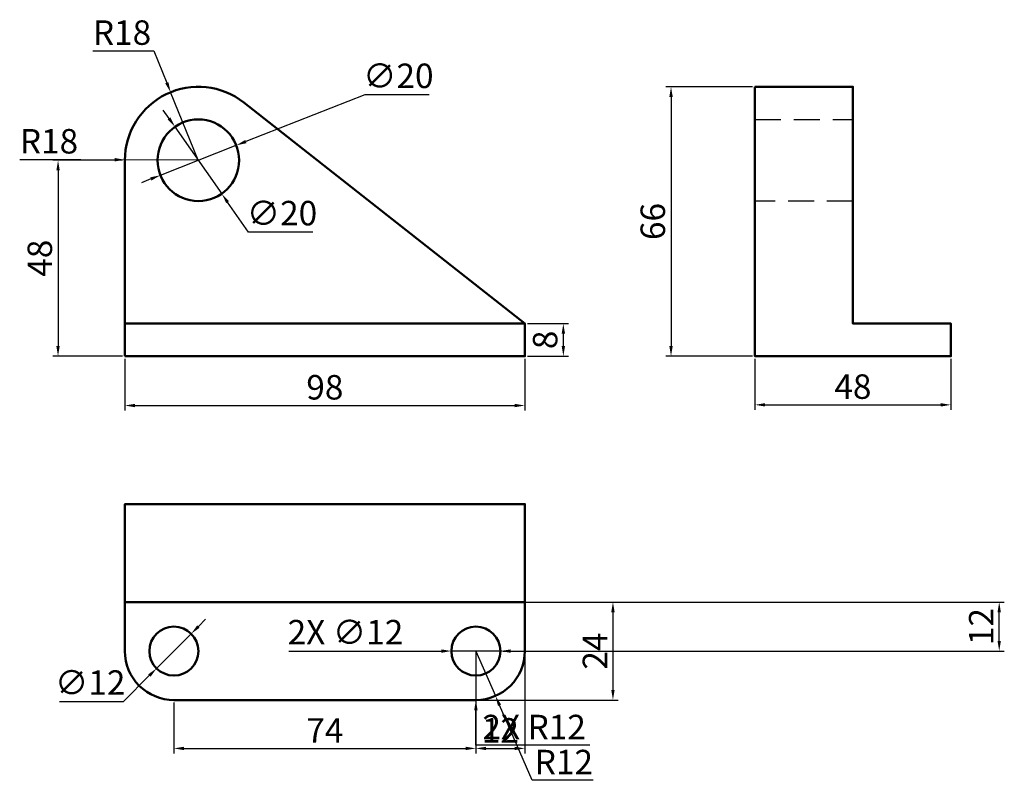
# Model space of a CAD drawing. Units: millimetres. Extents: x 6 to 247, y 96 to 282.
import ezdxf

# ---------------------------------------------------------------- set-up
doc = ezdxf.new("R2010")
doc.units = ezdxf.units.MM
doc.linetypes.add('HIDDEN', pattern=[9.525, 6.35, -3.175])
for name, color, linetype, lineweight in [('M-DIMS', 2, 'Continuous', 25), ('M-HIDN', 3, 'HIDDEN', 25), ('M-OUTL', 7, 'Continuous', 50)]:
    doc.layers.add(name, color=color, linetype=linetype, lineweight=lineweight)
doc.styles.get("Standard").update_dxf_attribs({"font": 'arial.ttf'})
doc.dimstyles.new('ISO-25', dxfattribs={"dimtxt": 6, "dimasz": 2.5, "dimexe": 1.25, "dimexo": 0.625, "dimtad": 1, "dimtoh": 1, "dimdec": 0, "dimtxsty": 'Standard', "dimcen": 2.5, "dimadec": 0, "dimazin": 0, "dimtfac": 1, "dimtdec": 0, "dimtmove": 0, "dimatfit": 3, "dimfxl": 1, "dimarcsym": 0})

# ---------------------------------------------------------------- blocks, each defined once
blk = doc.blocks.new('*D1')
at = {"layer": 'Defpoints', "color": 0, "transparency": 16777216}
for p in [(31.61, 247.68), (15.24, 199.68), (31.61, 199.68)]:
    blk.add_point(p, dxfattribs=at)
at = {"layer": 'M-DIMS', "color": 0, "lineweight": -2, "transparency": 16777216}
for p, q in [((30.99, 247.68), (13.99, 247.68)), ((15.24, 245.18), (15.24, 202.18)), ((30.99, 199.68), (13.99, 199.68))]:
    blk.add_line(p, q, dxfattribs=at)
at = {"layer": 'M-DIMS', "color": 0, "transparency": 16777216}
for points in [[(14.82, 245.18), (15.65, 245.18), (15.24, 247.68)], [(14.82, 202.18), (15.65, 202.18), (15.24, 199.68)]]:
    blk.add_solid(points, dxfattribs=at)
at = {"layer": 'M-DIMS', "color": 0, "transparency": 16777216, "insert": (11.55, 223.68), "char_height": 6, "attachment_point": 5, "rotation": 90}
blk.add_mtext('48', dxfattribs=at)
blk = doc.blocks.new('*D2')
at = {"layer": 'Defpoints', "color": 0, "transparency": 16777216}
for p in [(31.61, 199.68), (129.61, 199.68), (129.61, 187.6)]:
    blk.add_point(p, dxfattribs=at)
at = {"layer": 'M-DIMS', "color": 0, "lineweight": -2, "transparency": 16777216}
for p, q in [((31.61, 199.05), (31.61, 186.35)), ((129.61, 199.05), (129.61, 186.35)), ((34.11, 187.6), (127.11, 187.6))]:
    blk.add_line(p, q, dxfattribs=at)
at = {"layer": 'M-DIMS', "color": 0, "transparency": 16777216}
for points in [[(34.11, 188.01), (34.11, 187.18), (31.61, 187.6)], [(127.11, 188.01), (127.11, 187.18), (129.61, 187.6)]]:
    blk.add_solid(points, dxfattribs=at)
at = {"layer": 'M-DIMS', "color": 0, "transparency": 16777216, "insert": (80.61, 191.29), "char_height": 6, "attachment_point": 5}
blk.add_mtext('98', dxfattribs=at)
blk = doc.blocks.new('*D3')
at = {"layer": 'Defpoints', "color": 0, "transparency": 16777216}
for p in [(185.99, 265.68), (165.43, 199.68), (185.99, 199.68)]:
    blk.add_point(p, dxfattribs=at)
at = {"layer": 'M-DIMS', "color": 0, "lineweight": -2, "transparency": 16777216}
for p, q in [((185.36, 265.68), (164.18, 265.68)), ((165.43, 263.18), (165.43, 202.18)), ((185.36, 199.68), (164.18, 199.68))]:
    blk.add_line(p, q, dxfattribs=at)
at = {"layer": 'M-DIMS', "color": 0, "transparency": 16777216}
for points in [[(165.01, 263.18), (165.85, 263.18), (165.43, 265.68)], [(165.01, 202.18), (165.85, 202.18), (165.43, 199.68)]]:
    blk.add_solid(points, dxfattribs=at)
at = {"layer": 'M-DIMS', "color": 0, "transparency": 16777216, "insert": (161.74, 232.68), "char_height": 6, "attachment_point": 5, "rotation": 90}
blk.add_mtext('66', dxfattribs=at)
blk = doc.blocks.new('*D4')
at = {"layer": 'Defpoints', "color": 0, "transparency": 16777216}
for p in [(185.99, 199.68), (233.99, 199.68), (233.99, 187.76)]:
    blk.add_point(p, dxfattribs=at)
at = {"layer": 'M-DIMS', "color": 0, "lineweight": -2, "transparency": 16777216}
for p, q in [((185.99, 199.05), (185.99, 186.51)), ((233.99, 199.05), (233.99, 186.51)), ((188.49, 187.76), (231.49, 187.76))]:
    blk.add_line(p, q, dxfattribs=at)
at = {"layer": 'M-DIMS', "color": 0, "transparency": 16777216}
for points in [[(188.49, 188.18), (188.49, 187.35), (185.99, 187.76)], [(231.49, 188.18), (231.49, 187.35), (233.99, 187.76)]]:
    blk.add_solid(points, dxfattribs=at)
at = {"layer": 'M-DIMS', "color": 0, "transparency": 16777216, "insert": (209.99, 191.45), "char_height": 6, "attachment_point": 5}
blk.add_mtext('48', dxfattribs=at)
blk = doc.blocks.new('*D5')
at = {"layer": 'Defpoints', "color": 0, "transparency": 16777216}
for p in [(80.61, 139.44), (80.61, 115.44), (151.2, 115.44)]:
    blk.add_point(p, dxfattribs=at)
at = {"layer": 'M-DIMS', "color": 0, "lineweight": -2, "transparency": 16777216}
for p, q in [((81.24, 139.44), (152.45, 139.44)), ((151.2, 136.94), (151.2, 117.94)), ((81.24, 115.44), (152.45, 115.44))]:
    blk.add_line(p, q, dxfattribs=at)
at = {"layer": 'M-DIMS', "color": 0, "transparency": 16777216}
for points in [[(150.78, 136.94), (151.61, 136.94), (151.2, 139.44)], [(150.78, 117.94), (151.61, 117.94), (151.2, 115.44)]]:
    blk.add_solid(points, dxfattribs=at)
at = {"layer": 'M-DIMS', "color": 0, "transparency": 16777216, "insert": (147.56, 127.44), "char_height": 6, "attachment_point": 5, "rotation": 90}
blk.add_mtext('24', dxfattribs=at)
blk = doc.blocks.new('*D6')
at = {"layer": 'Defpoints', "color": 0, "transparency": 16777216}
for p in [(129.61, 207.68), (129.61, 199.68), (139.04, 199.68)]:
    blk.add_point(p, dxfattribs=at)
at = {"layer": 'M-DIMS', "color": 0, "lineweight": -2, "transparency": 16777216}
for p, q in [((130.24, 207.68), (140.29, 207.68)), ((139.04, 205.18), (139.04, 202.18)), ((130.24, 199.68), (140.29, 199.68))]:
    blk.add_line(p, q, dxfattribs=at)
at = {"layer": 'M-DIMS', "color": 0, "transparency": 16777216}
for points in [[(138.63, 205.18), (139.46, 205.18), (139.04, 207.68)], [(138.63, 202.18), (139.46, 202.18), (139.04, 199.68)]]:
    blk.add_solid(points, dxfattribs=at)
at = {"layer": 'M-DIMS', "color": 0, "transparency": 16777216, "insert": (135.36, 203.68), "char_height": 6, "attachment_point": 5, "rotation": 90}
blk.add_mtext('8', dxfattribs=at)
blk = doc.blocks.new('*D7')
at = {"layer": 'Defpoints', "color": 0, "transparency": 16777216}
for p in [(58.92, 251.34), (40.31, 244.01)]:
    blk.add_point(p, dxfattribs=at)
at = {"layer": 'M-DIMS', "color": 0, "lineweight": -2, "transparency": 16777216}
for p, q in [((90.44, 263.74), (61.25, 252.25)), ((106.17, 263.74), (90.44, 263.74)), ((40.31, 244.01), (58.92, 251.34)), ((37.98, 243.1), (35.66, 242.18))]:
    blk.add_line(p, q, dxfattribs=at)
at = {"layer": 'M-DIMS', "color": 0, "transparency": 16777216}
for points in [[(61.09, 252.64), (61.4, 251.87), (58.92, 251.34)], [(37.83, 243.49), (38.14, 242.71), (40.31, 244.01)]]:
    blk.add_solid(points, dxfattribs=at)
at = {"layer": 'M-DIMS', "color": 0, "transparency": 16777216, "insert": (98.61, 267.59), "char_height": 6, "attachment_point": 5}
blk.add_mtext('∅20', dxfattribs=at)
blk = doc.blocks.new('*D8')
at = {"layer": 'Defpoints', "color": 0, "transparency": 16777216}
for p in [(42.83, 264.35), (49.61, 247.68)]:
    blk.add_point(p, dxfattribs=at)
at = {"layer": 'M-DIMS', "color": 0, "lineweight": -2, "transparency": 16777216}
for p, q in [((23.73, 274.49), (38.71, 274.49)), ((38.71, 274.49), (41.89, 266.67)), ((49.61, 247.68), (42.83, 264.35))]:
    blk.add_line(p, q, dxfattribs=at)
at = {"layer": 'M-DIMS', "color": 0, "transparency": 16777216}
blk.add_solid([(42.28, 266.82), (41.5, 266.51), (42.83, 264.35)], dxfattribs=at)
at = {"layer": 'M-DIMS', "color": 0, "transparency": 16777216, "insert": (30.91, 278.18), "char_height": 6, "attachment_point": 5}
blk.add_mtext('R18', dxfattribs=at)
blk = doc.blocks.new('*D9')
at = {"layer": 'Defpoints', "color": 0, "transparency": 16777216}
for p in [(47.86, 131.68), (39.37, 123.2)]:
    blk.add_point(p, dxfattribs=at)
at = {"layer": 'M-DIMS', "color": 0, "lineweight": -2, "transparency": 16777216}
for p, q in [((49.63, 133.45), (51.39, 135.22)), ((47.86, 131.68), (39.37, 123.2)), ((31.27, 115.09), (37.6, 121.43)), ((15.58, 115.09), (31.27, 115.09))]:
    blk.add_line(p, q, dxfattribs=at)
at = {"layer": 'M-DIMS', "color": 0, "transparency": 16777216}
for points in [[(49.33, 133.74), (49.92, 133.15), (47.86, 131.68)], [(37.31, 121.72), (37.9, 121.13), (39.37, 123.2)]]:
    blk.add_solid(points, dxfattribs=at)
at = {"layer": 'M-DIMS', "color": 0, "transparency": 16777216, "insert": (23.11, 118.95), "char_height": 6, "attachment_point": 5}
blk.add_mtext('∅12', dxfattribs=at)
blk = doc.blocks.new('*D10')
at = {"layer": 'Defpoints', "color": 0, "transparency": 16777216}
for p in [(117.61, 127.44), (122.41, 116.44)]:
    blk.add_point(p, dxfattribs=at)
at = {"layer": 'M-DIMS', "color": 0, "lineweight": -2, "transparency": 16777216}
for p, q in [((117.61, 127.44), (122.41, 116.44)), ((131.41, 95.83), (123.41, 114.15)), ((146.31, 95.83), (131.41, 95.83))]:
    blk.add_line(p, q, dxfattribs=at)
at = {"layer": 'M-DIMS', "color": 0, "transparency": 16777216}
blk.add_solid([(123.8, 114.32), (123.03, 113.98), (122.41, 116.44)], dxfattribs=at)
at = {"layer": 'M-DIMS', "color": 0, "transparency": 16777216, "insert": (139.17, 99.47), "char_height": 6, "attachment_point": 5}
blk.add_mtext('R12', dxfattribs=at)
blk = doc.blocks.new('BASE-HOLE-D12')
blk.add_circle((6, 6), 6)
blk = doc.blocks.new('*D12')
at = {"layer": 'Defpoints', "color": 0, "transparency": 16777216}
for p in [(117.61, 127.44), (129.61, 127.44), (129.61, 103.59)]:
    blk.add_point(p, dxfattribs=at)
at = {"layer": 'M-DIMS', "color": 0, "lineweight": -2, "transparency": 16777216}
for p, q in [((117.61, 126.81), (117.61, 102.34)), ((129.61, 126.81), (129.61, 102.34)), ((120.11, 103.59), (127.11, 103.59))]:
    blk.add_line(p, q, dxfattribs=at)
at = {"layer": 'M-DIMS', "color": 0, "transparency": 16777216}
for points in [[(120.11, 104), (120.11, 103.17), (117.61, 103.59)], [(127.11, 104), (127.11, 103.17), (129.61, 103.59)]]:
    blk.add_solid(points, dxfattribs=at)
at = {"layer": 'M-DIMS', "color": 0, "transparency": 16777216, "insert": (123.61, 107.23), "char_height": 6, "attachment_point": 5}
blk.add_mtext('12', dxfattribs=at)
blk = doc.blocks.new('*D13')
at = {"layer": 'Defpoints', "color": 0, "transparency": 16777216}
for p in [(117.61, 127.44), (43.61, 115.44), (117.61, 103.59)]:
    blk.add_point(p, dxfattribs=at)
at = {"layer": 'M-DIMS', "color": 0, "lineweight": -2, "transparency": 16777216}
for p, q in [((117.61, 126.81), (117.61, 102.34)), ((43.61, 114.81), (43.61, 102.34)), ((46.11, 103.59), (115.11, 103.59))]:
    blk.add_line(p, q, dxfattribs=at)
at = {"layer": 'M-DIMS', "color": 0, "transparency": 16777216}
for points in [[(46.11, 104), (46.11, 103.17), (43.61, 103.59)], [(115.11, 104), (115.11, 103.17), (117.61, 103.59)]]:
    blk.add_solid(points, dxfattribs=at)
at = {"layer": 'M-DIMS', "color": 0, "transparency": 16777216, "insert": (80.61, 107.21), "char_height": 6, "attachment_point": 5}
blk.add_mtext('74', dxfattribs=at)
blk = doc.blocks.new('*D14')
at = {"layer": 'Defpoints', "color": 0, "transparency": 16777216}
for p in [(129.61, 139.44), (245.84, 139.44), (123.61, 127.44)]:
    blk.add_point(p, dxfattribs=at)
at = {"layer": 'M-DIMS', "color": 0, "lineweight": -2, "transparency": 16777216}
for p, q in [((130.24, 139.44), (247.09, 139.44)), ((245.84, 129.94), (245.84, 136.94)), ((124.24, 127.44), (247.09, 127.44))]:
    blk.add_line(p, q, dxfattribs=at)
at = {"layer": 'M-DIMS', "color": 0, "transparency": 16777216}
for points in [[(245.42, 136.94), (246.25, 136.94), (245.84, 139.44)], [(245.42, 129.94), (246.25, 129.94), (245.84, 127.44)]]:
    blk.add_solid(points, dxfattribs=at)
at = {"layer": 'M-DIMS', "color": 0, "transparency": 16777216, "insert": (242.2, 133.44), "char_height": 6, "attachment_point": 5, "rotation": 90}
blk.add_mtext('12', dxfattribs=at)
blk = doc.blocks.new('*D15')
at = {"layer": 'Defpoints', "color": 0, "transparency": 16777216}
for p in [(31.62, 247.8), (49.61, 247.68)]:
    blk.add_point(p, dxfattribs=at)
at = {"layer": 'M-DIMS', "color": 0, "lineweight": -2, "transparency": 16777216}
for p, q in [((5.84, 247.87), (20.82, 247.87)), ((20.82, 247.87), (29.12, 247.82)), ((49.61, 247.68), (31.62, 247.8))]:
    blk.add_line(p, q, dxfattribs=at)
at = {"layer": 'M-DIMS', "color": 0, "transparency": 16777216}
blk.add_solid([(29.12, 248.23), (29.11, 247.4), (31.62, 247.8)], dxfattribs=at)
at = {"layer": 'M-DIMS', "color": 0, "transparency": 16777216, "insert": (13.02, 251.56), "char_height": 6, "attachment_point": 5}
blk.add_mtext('R18', dxfattribs=at)
blk = doc.blocks.new('*D16')
at = {"layer": 'Defpoints', "color": 0, "transparency": 16777216}
for p in [(43.88, 255.87), (55.35, 239.48)]:
    blk.add_point(p, dxfattribs=at)
at = {"layer": 'M-DIMS', "color": 0, "lineweight": -2, "transparency": 16777216}
for p, q in [((42.45, 257.92), (41.02, 259.97)), ((43.88, 255.87), (55.35, 239.48)), ((61.92, 230.09), (56.78, 237.43)), ((77.65, 230.09), (61.92, 230.09))]:
    blk.add_line(p, q, dxfattribs=at)
at = {"layer": 'M-DIMS', "color": 0, "transparency": 16777216}
for points in [[(42.79, 258.16), (42.11, 257.68), (43.88, 255.87)], [(57.12, 237.67), (56.44, 237.2), (55.35, 239.48)]]:
    blk.add_solid(points, dxfattribs=at)
at = {"layer": 'M-DIMS', "color": 0, "transparency": 16777216, "insert": (70.1, 233.95), "char_height": 6, "attachment_point": 5}
blk.add_mtext('∅20', dxfattribs=at)
blk = doc.blocks.new('*D17')
at = {"layer": 'Defpoints', "color": 0, "transparency": 16777216}
for p in [(117.61, 127.44), (117.62, 115.44)]:
    blk.add_point(p, dxfattribs=at)
at = {"layer": 'M-DIMS', "color": 0, "lineweight": -2, "transparency": 16777216}
for p, q in [((117.61, 127.44), (117.62, 115.44)), ((117.62, 104.41), (117.62, 112.94)), ((145.51, 104.41), (117.62, 104.41))]:
    blk.add_line(p, q, dxfattribs=at)
at = {"layer": 'M-DIMS', "color": 0, "transparency": 16777216}
blk.add_solid([(118.03, 112.94), (117.2, 112.94), (117.62, 115.44)], dxfattribs=at)
at = {"layer": 'M-DIMS', "color": 0, "transparency": 16777216, "insert": (131.88, 108.05), "char_height": 6, "attachment_point": 5}
blk.add_mtext('2X R12', dxfattribs=at)
blk = doc.blocks.new('*D18')
at = {"layer": 'Defpoints', "color": 0, "transparency": 16777216}
for p in [(111.61, 127.44), (123.61, 127.44)]:
    blk.add_point(p, dxfattribs=at)
at = {"layer": 'M-DIMS', "color": 0, "lineweight": -2, "transparency": 16777216}
for p, q in [((71.79, 127.44), (100.15, 127.44)), ((100.15, 127.44), (109.11, 127.44)), ((123.61, 127.44), (111.61, 127.44)), ((126.11, 127.44), (128.61, 127.44))]:
    blk.add_line(p, q, dxfattribs=at)
at = {"layer": 'M-DIMS', "color": 0, "transparency": 16777216}
for points in [[(109.11, 127.85), (109.11, 127.02), (111.61, 127.44)], [(126.11, 127.85), (126.11, 127.02), (123.61, 127.44)]]:
    blk.add_solid(points, dxfattribs=at)
at = {"layer": 'M-DIMS', "color": 0, "transparency": 16777216, "insert": (85.66, 131.29), "char_height": 6, "attachment_point": 5}
blk.add_mtext('2X ∅12', dxfattribs=at)

msp = doc.modelspace()

# ---------------------------------------------------------------- linework, layer by layer
at = {"layer": 'M-HIDN'}
msp.add_lwpolyline([(185.99, 257.68), (209.99, 257.68), (209.99, 237.68), (185.99, 237.68)], dxfattribs=at)
at = {"layer": 'M-OUTL'}
for p, q in [((31.61, 207.68), (129.61, 207.68)), ((31.61, 139.44), (129.61, 139.44))]:
    msp.add_line(p, q, dxfattribs=at)
for points in [[(31.61, 199.68), (31.61, 247.68, -0.625931), (60.74, 261.83), (129.61, 207.68), (129.61, 199.68)], [(43.61, 115.44), (117.61, 115.44, 0.414214), (129.61, 127.44), (129.61, 163.44), (31.61, 163.44), (31.61, 127.44, 0.414214)]]:
    msp.add_lwpolyline(points, format="xyb", close=True, dxfattribs=at)
msp.add_lwpolyline([(185.99, 265.68), (209.99, 265.68), (209.99, 207.68), (233.99, 207.68), (233.99, 199.68), (185.99, 199.68)], close=True, dxfattribs=at)
msp.add_circle((49.61, 247.68), 10, dxfattribs=at)

# ---------------------------------------------------------------- block references
for p in [(37.62, 121.44), (111.61, 121.44)]:
    msp.add_blockref('BASE-HOLE-D12', p, dxfattribs=at)

# ---------------------------------------------------------------- dimensions: what is measured, and where the dimension line sits
at = {"layer": 'M-DIMS'}
for center, mpoint, override, picture, middle in [((49.61, 247.68), (42.83, 264.35), {"dimclrd": 0, "dimclre": 0, "dimclrt": 0}, '*D8', (30.91, 274.49)), ((49.61, 247.68), (31.62, 247.8), {"dimdec": 0, "dimlfac": 1, "dimrnd": 0, "dimzin": 0, "dimdsep": 46, "dimlunit": 2}, '*D15', (20.82, 247.87)), ((117.61, 127.44), (122.41, 116.44), {"dimclrd": 0, "dimclre": 0, "dimclrt": 0}, '*D10', (139.17, 95.83))]:
    dim = msp.add_radius_dim(center=center, mpoint=mpoint, dimstyle='ISO-25', override=override, dxfattribs=at)
    dim.commit()
    dim.dimension.update_dxf_attribs({"geometry": picture, "text_midpoint": middle, "dimtype": 164})
for p1, p2, override, picture, middle in [((40.31, 244.01), (58.92, 251.34), {"dimclrd": 0, "dimclre": 0, "dimclrt": 0}, '*D7', (98.61, 263.74)), ((43.88, 255.87), (55.35, 239.48), {"dimdec": 0, "dimlfac": 1, "dimrnd": 0, "dimzin": 0, "dimdsep": 46, "dimlunit": 2}, '*D16', (70.1, 230.09))]:
    dim = msp.add_diameter_dim_2p(p1=p1, p2=p2, dimstyle='ISO-25', override=override, dxfattribs=at)
    dim.commit()
    dim.dimension.update_dxf_attribs({"geometry": picture, "text_midpoint": middle, "dimtype": 163})
for base, p1, p2, override, picture, middle in [((165.43, 199.68), (185.99, 265.68), (185.99, 199.68), {"dimclrd": 0, "dimclre": 0, "dimclrt": 0}, '*D3', (161.74, 232.68)), ((15.24, 199.68), (31.61, 247.68), (31.61, 199.68), {"dimclrd": 0, "dimclre": 0, "dimclrt": 0}, '*D1', (11.55, 223.68)), ((139.04, 199.68), (129.61, 207.68), (129.61, 199.68), {"dimclrd": 0, "dimclre": 0, "dimclrt": 0}, '*D6', (135.36, 203.68)), ((151.2, 115.44), (80.61, 139.44), (80.61, 115.44), {"dimclrd": 0, "dimclre": 0, "dimclrt": 0}, '*D5', (147.56, 127.44)), ((245.84, 139.44), (123.61, 127.44), (129.61, 139.44), {"dimdec": 0, "dimlfac": 1, "dimrnd": 0, "dimzin": 0, "dimdsep": 46, "dimlunit": 2}, '*D14', (242.2, 133.44))]:
    dim = msp.add_linear_dim(base=base, p1=p1, p2=p2, angle=90, dimstyle='ISO-25', override=override, dxfattribs=at)
    dim.commit()
    dim.dimension.update_dxf_attribs({"geometry": picture, "text_midpoint": middle})
for base, p1, p2, override, picture, middle in [((129.61, 187.6), (31.61, 199.68), (129.61, 199.68), {"dimclrd": 0, "dimclre": 0, "dimclrt": 0}, '*D2', (80.61, 191.29)), ((233.99, 187.76), (185.99, 199.68), (233.99, 199.68), {"dimclrd": 0, "dimclre": 0, "dimclrt": 0}, '*D4', (209.99, 191.45)), ((117.61, 103.59), (43.61, 115.44), (117.61, 127.44), {"dimdec": 0, "dimlfac": 1, "dimrnd": 0, "dimzin": 0, "dimdsep": 46, "dimlunit": 2}, '*D13', (80.61, 107.21)), ((129.61, 103.59), (117.61, 127.44), (129.61, 127.44), {"dimdec": 0, "dimlfac": 1, "dimrnd": 0, "dimzin": 0, "dimdsep": 46, "dimlunit": 2}, '*D12', (123.61, 107.23))]:
    dim = msp.add_linear_dim(base=base, p1=p1, p2=p2, dimstyle='ISO-25', override=override, dxfattribs=at)
    dim.commit()
    dim.dimension.update_dxf_attribs({"geometry": picture, "text_midpoint": middle})
dim = msp.add_diameter_dim_2p(p1=(123.61, 127.44), p2=(111.61, 127.44), text='2X <>', dimstyle='ISO-25', override={"dimdec": 0, "dimlfac": 1, "dimrnd": 0, "dimzin": 0, "dimdsep": 46, "dimlunit": 2}, dxfattribs=at)
dim.commit()
dim.dimension.update_dxf_attribs({"geometry": '*D18', "text_midpoint": (100.15, 127.44), "dimtype": 163})
dim = msp.add_diameter_dim_2p(p1=(47.86, 131.68), p2=(39.37, 123.2), dimstyle='ISO-25', override={"dimclrd": 0, "dimclre": 0, "dimclrt": 0}, dxfattribs=at)
dim.commit()
dim.dimension.update_dxf_attribs({"geometry": '*D9', "text_midpoint": (23.11, 118.95)})
dim = msp.add_radius_dim(center=(117.61, 127.44), mpoint=(117.62, 115.44), text='2X <>', dimstyle='ISO-25', override={"dimdec": 0, "dimlfac": 1, "dimrnd": 0, "dimzin": 0, "dimdsep": 46, "dimlunit": 2}, dxfattribs=at)
dim.commit()
dim.dimension.update_dxf_attribs({"geometry": '*D17', "text_midpoint": (131.88, 108.05)})

doc.saveas('drawing.dxf')
